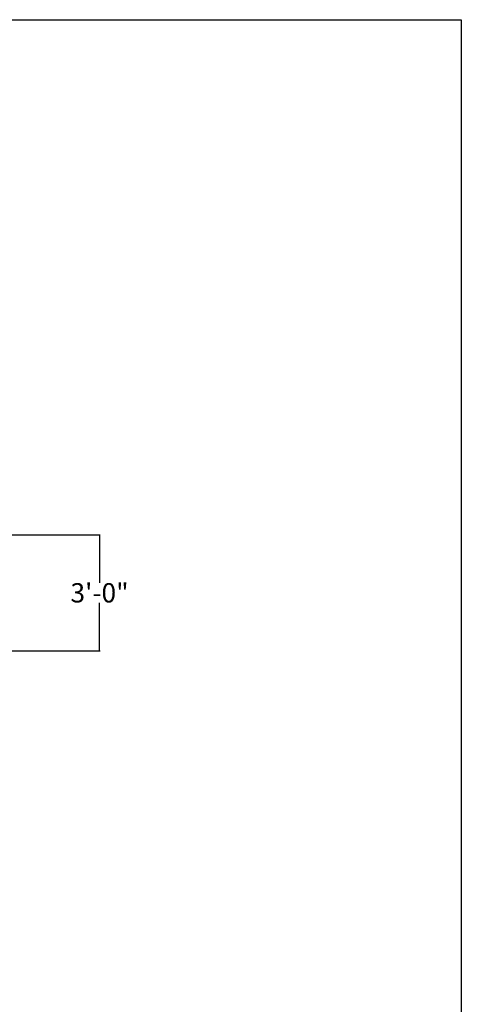
# Model space of a CAD drawing. Units: inches. Extents: x 2552 to 3196, y 4736 to 5443.
# Tile 8 of 8: x 3058 to 3196, y 5136 to 5443. Entities that reach past the tile are written whole.
import ezdxf

# ---------------------------------------------------------------- set-up
doc = ezdxf.new("R2010")
doc.units = ezdxf.units.IN
doc.header["$MEASUREMENT"] = 0
doc.layers.add('A-ANNO-DIMS', color=2, linetype='Continuous', lineweight=18)
doc.layers.add('A-ANNO-TTLB', color=7, linetype='Continuous', lineweight=25)
doc.styles.get("Standard").update_dxf_attribs({"font": 'arial.ttf'})
doc.dimstyles.get("Standard").update_dxf_attribs({"dimtxt": 6, "dimasz": 0.18, "dimexe": 0.18, "dimexo": 0.0625, "dimgap": 0.09, "dimtad": 0, "dimtih": 1, "dimtoh": 1, "dimdec": 1, "dimzin": 0, "dimdsep": 46, "dimlunit": 3, "dimtxsty": 'Standard', "dimcen": 0.09, "dimadec": 0, "dimazin": 0, "dimtfac": 1, "dimtdec": 1, "dimtofl": 0, "dimtmove": 0, "dimatfit": 3, "dimfxl": 1, "dimtolj": 1, "dimtzin": 0, "dimarcsym": 0})

# ---------------------------------------------------------------- blocks, each defined once
blk = doc.blocks.new('*D44')
at = {"layer": 'A-ANNO-DIMS', "color": 0, "lineweight": -2, "transparency": 16777216}
for p, q in [((2889.29, 5282.32), (3083.39, 5282.32)), ((3083.21, 5282.14), (3083.21, 5267.47)), ((3083.21, 5246.5), (3083.21, 5261.16)), ((2904.72, 5246.32), (3083.39, 5246.32))]:
    blk.add_line(p, q, dxfattribs=at)
at = {"layer": 'A-ANNO-DIMS', "color": 0, "transparency": 16777216}
for points in [[(3083.18, 5282.14), (3083.24, 5282.14), (3083.21, 5282.32)], [(3083.18, 5246.5), (3083.24, 5246.5), (3083.21, 5246.32)]]:
    blk.add_solid(points, dxfattribs=at)
at = {"layer": 'Defpoints', "color": 0, "transparency": 16777216}
for p in [(2889.22, 5282.32), (2904.66, 5246.32), (3083.21, 5246.32)]:
    blk.add_point(p, dxfattribs=at)
at = {"layer": 'A-ANNO-DIMS', "color": 0, "transparency": 16777216, "insert": (3083.21, 5264.32), "char_height": 6, "attachment_point": 5}
blk.add_mtext('\\A1;3\'-0"', dxfattribs=at)

msp = doc.modelspace()

# ---------------------------------------------------------------- linework, layer by layer
at = {"layer": 'A-ANNO-TTLB'}
msp.add_lwpolyline([(2551.65, 5442.6), (3195.75, 5442.6), (3195.75, 4736.32), (2551.65, 4736.32)], close=True, dxfattribs=at)

# ---------------------------------------------------------------- dimensions: what is measured, and where the dimension line sits
at = {"layer": 'A-ANNO-DIMS'}
dim = msp.add_linear_dim(base=(3083.21, 5246.32), p1=(2889.22, 5282.32), p2=(2904.66, 5246.32), angle=90, dimstyle='Standard', override={"dimdec": 1, "dimlfac": 1, "dimrnd": 0, "dimzin": 1, "dimdsep": 46, "dimlunit": 4, "dimfrac": 2}, dxfattribs=at)
dim.commit()
dim.dimension.update_dxf_attribs({"geometry": '*D44', "text_midpoint": (3083.21, 5264.32)})

doc.saveas('drawing.dxf')
